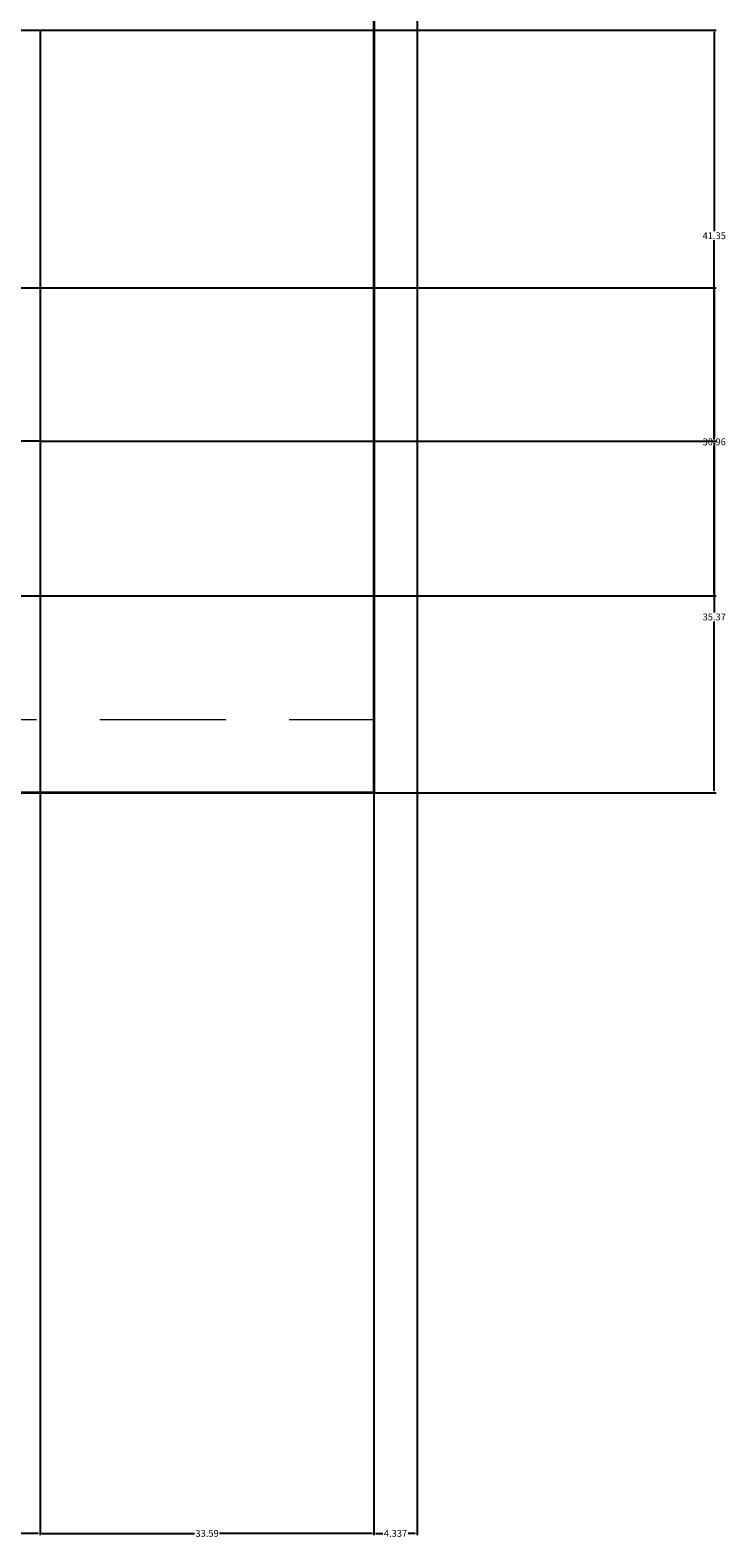
# Model space of a CAD drawing. Units: inches. Extents: x -145 to 510, y 5 to 386.
# Tile 18 of 25: x 440 to 510, y 5 to 157. Entities that reach past the tile are written whole.
import ezdxf

# ---------------------------------------------------------------- set-up
doc = ezdxf.new("R2010")
doc.units = ezdxf.units.IN
doc.header["$MEASUREMENT"] = 0
doc.linetypes.add('DASHED', pattern=[19.05, 12.7, -6.35])
for name, color, linetype, lineweight in [('A-ANNO-DIMS', 2, 'Continuous', 18), ('A-ELEV', 7, 'Continuous', 35), ('A-ELEV-HIDN', 8, 'DASHED', 18), ('A-GLAZ', 4, 'Continuous', 25)]:
    doc.layers.add(name, color=color, linetype=linetype, lineweight=lineweight)
doc.styles.get("Standard").update_dxf_attribs({"font": 'arial.ttf'})
doc.dimstyles.get("Standard").update_dxf_attribs({"dimtxt": 0.6875, "dimasz": 0.18, "dimexe": 0.18, "dimexo": 0.0625, "dimgap": 0.09, "dimtad": 0, "dimtih": 1, "dimtoh": 1, "dimdec": 4, "dimzin": 0, "dimdsep": 46, "dimlunit": 4, "dimtxsty": 'Standard', "dimcen": 0.09, "dimadec": 0, "dimazin": 0, "dimtfac": 1, "dimtdec": 4, "dimtofl": 0, "dimtmove": 0, "dimatfit": 3, "dimfxl": 1, "dimtolj": 1, "dimtzin": 0, "dimarcsym": 0})

# ---------------------------------------------------------------- blocks, each defined once
blk = doc.blocks.new('*D12')
at = {"layer": 'A-ANNO-DIMS', "color": 0, "lineweight": -2, "transparency": 16777216}
for p, q in [((353.23, 115.19), (353.23, 5.19)), ((440.9, 115.19), (440.9, 5.19)), ((353.41, 5.37), (395.82, 5.37)), ((440.72, 5.37), (398.32, 5.37))]:
    blk.add_line(p, q, dxfattribs=at)
at = {"layer": 'A-ANNO-DIMS', "color": 0, "transparency": 16777216}
for points in [[(353.41, 5.4), (353.41, 5.34), (353.23, 5.37)], [(440.72, 5.4), (440.72, 5.34), (440.9, 5.37)]]:
    blk.add_solid(points, dxfattribs=at)
at = {"layer": 'Defpoints', "color": 0, "transparency": 16777216}
for p in [(353.23, 115.26), (440.9, 115.26), (440.9, 5.37)]:
    blk.add_point(p, dxfattribs=at)
at = {"layer": 'A-ANNO-DIMS', "color": 0, "transparency": 16777216, "insert": (397.07, 5.37), "char_height": 0.688, "attachment_point": 5}
blk.add_mtext('\\A1;87.67', dxfattribs=at)
blk = doc.blocks.new('*D13')
at = {"layer": 'A-ANNO-DIMS', "color": 0, "lineweight": -2, "transparency": 16777216}
for p, q in [((440.9, 115.19), (440.9, 5.19)), ((474.49, 79.83), (474.49, 5.19)), ((441.08, 5.37), (456.44, 5.37)), ((474.31, 5.37), (458.95, 5.37))]:
    blk.add_line(p, q, dxfattribs=at)
at = {"layer": 'A-ANNO-DIMS', "color": 0, "transparency": 16777216}
for points in [[(441.08, 5.4), (441.08, 5.34), (440.9, 5.37)], [(474.31, 5.4), (474.31, 5.34), (474.49, 5.37)]]:
    blk.add_solid(points, dxfattribs=at)
at = {"layer": 'Defpoints', "color": 0, "transparency": 16777216}
for p in [(440.9, 115.26), (474.49, 79.89), (474.49, 5.37)]:
    blk.add_point(p, dxfattribs=at)
at = {"layer": 'A-ANNO-DIMS', "color": 0, "transparency": 16777216, "insert": (457.7, 5.37), "char_height": 0.688, "attachment_point": 5}
blk.add_mtext('\\A1;33.59', dxfattribs=at)
blk = doc.blocks.new('*D19')
at = {"layer": 'A-ANNO-DIMS', "color": 0, "lineweight": -2, "transparency": 16777216}
for p, q in [((478.76, 355.89), (-144.05, 355.89)), ((-143.87, 355.71), (-143.87, 218.33)), ((-143.87, 80.07), (-143.87, 217.45)), ((-114.04, 79.89), (-144.05, 79.89))]:
    blk.add_line(p, q, dxfattribs=at)
at = {"layer": 'A-ANNO-DIMS', "color": 0, "transparency": 16777216}
for points in [[(-143.9, 355.71), (-143.84, 355.71), (-143.87, 355.89)], [(-143.9, 80.07), (-143.84, 80.07), (-143.87, 79.89)]]:
    blk.add_solid(points, dxfattribs=at)
at = {"layer": 'Defpoints', "color": 0, "transparency": 16777216}
for p in [(-143.87, 355.89), (478.83, 355.89), (-113.97, 79.89)]:
    blk.add_point(p, dxfattribs=at)
at = {"layer": 'A-ANNO-DIMS', "color": 0, "transparency": 16777216, "insert": (-143.87, 217.89), "char_height": 0.688, "attachment_point": 5}
blk.add_mtext('\\A1;276', dxfattribs=at)
blk = doc.blocks.new('*D31')
at = {"layer": 'A-ANNO-DIMS', "color": 0, "lineweight": -2, "transparency": 16777216}
for p, q in [((440.96, 115.26), (508.91, 115.26)), ((508.73, 115.08), (508.73, 98.02)), ((508.73, 80.07), (508.73, 97.13)), ((474.55, 79.89), (508.91, 79.89))]:
    blk.add_line(p, q, dxfattribs=at)
at = {"layer": 'A-ANNO-DIMS', "color": 0, "transparency": 16777216}
for points in [[(508.7, 115.08), (508.76, 115.08), (508.73, 115.26)], [(508.7, 80.07), (508.76, 80.07), (508.73, 79.89)]]:
    blk.add_solid(points, dxfattribs=at)
at = {"layer": 'Defpoints', "color": 0, "transparency": 16777216}
for p in [(440.9, 115.26), (508.73, 115.26), (474.49, 79.89)]:
    blk.add_point(p, dxfattribs=at)
at = {"layer": 'A-ANNO-DIMS', "color": 0, "transparency": 16777216, "insert": (508.73, 97.57), "char_height": 0.688, "attachment_point": 5}
blk.add_mtext('\\A1;35.37', dxfattribs=at)
blk = doc.blocks.new('*D32')
at = {"layer": 'A-ANNO-DIMS', "color": 0, "lineweight": -2, "transparency": 16777216}
for p, q in [((440.96, 156.61), (508.91, 156.61)), ((508.73, 156.43), (508.73, 136.37)), ((508.73, 115.44), (508.73, 135.49)), ((440.96, 115.26), (508.91, 115.26))]:
    blk.add_line(p, q, dxfattribs=at)
at = {"layer": 'A-ANNO-DIMS', "color": 0, "transparency": 16777216}
for points in [[(508.7, 156.43), (508.76, 156.43), (508.73, 156.61)], [(508.7, 115.44), (508.76, 115.44), (508.73, 115.26)]]:
    blk.add_solid(points, dxfattribs=at)
at = {"layer": 'Defpoints', "color": 0, "transparency": 16777216}
for p in [(440.9, 156.61), (508.73, 156.61), (440.9, 115.26)]:
    blk.add_point(p, dxfattribs=at)
at = {"layer": 'A-ANNO-DIMS', "color": 0, "transparency": 16777216, "insert": (508.73, 135.93), "char_height": 0.688, "attachment_point": 5}
blk.add_mtext('\\A1;41.35', dxfattribs=at)
blk = doc.blocks.new('*D49')
at = {"layer": 'A-ANNO-DIMS', "color": 0, "lineweight": -2, "transparency": 16777216}
for p, q in [((474.49, 223.83), (474.49, 5.19)), ((478.83, 223.83), (478.83, 5.19)), ((474.67, 5.37), (475.39, 5.37)), ((478.65, 5.37), (477.92, 5.37))]:
    blk.add_line(p, q, dxfattribs=at)
at = {"layer": 'A-ANNO-DIMS', "color": 0, "transparency": 16777216}
for points in [[(474.67, 5.4), (474.67, 5.34), (474.49, 5.37)], [(478.65, 5.4), (478.65, 5.34), (478.83, 5.37)]]:
    blk.add_solid(points, dxfattribs=at)
at = {"layer": 'Defpoints', "color": 0, "transparency": 16777216}
for p in [(474.49, 223.89), (478.83, 223.89), (478.83, 5.37)]:
    blk.add_point(p, dxfattribs=at)
at = {"layer": 'A-ANNO-DIMS', "color": 0, "transparency": 16777216, "insert": (476.66, 5.37), "char_height": 0.688, "attachment_point": 5}
blk.add_mtext('\\A1;4.337', dxfattribs=at)
blk = doc.blocks.new('*D58')
at = {"layer": 'A-ANNO-DIMS', "color": 0, "lineweight": -2, "transparency": 16777216}
for p, q in [((265.82, 130.67), (508.91, 130.67)), ((508.73, 130.49), (508.73, 115.63)), ((508.73, 99.89), (508.73, 114.75)), ((265.82, 99.71), (508.91, 99.71))]:
    blk.add_line(p, q, dxfattribs=at)
at = {"layer": 'A-ANNO-DIMS', "color": 0, "transparency": 16777216}
for points in [[(508.7, 130.49), (508.76, 130.49), (508.73, 130.67)], [(508.7, 99.89), (508.76, 99.89), (508.73, 99.71)]]:
    blk.add_solid(points, dxfattribs=at)
at = {"layer": 'Defpoints', "color": 0, "transparency": 16777216}
for p in [(265.76, 130.67), (508.73, 130.67), (265.76, 99.71)]:
    blk.add_point(p, dxfattribs=at)
at = {"layer": 'A-ANNO-DIMS', "color": 0, "transparency": 16777216, "insert": (508.73, 115.19), "char_height": 0.688, "attachment_point": 5}
blk.add_mtext('\\A1;30.96', dxfattribs=at)

msp = doc.modelspace()

# ---------------------------------------------------------------- linework, layer by layer
at = {"layer": 'A-ELEV'}
for p, q in [((474.4893, 223.8905), (474.4893, 79.8905)), ((474.4893, 79.8905), (392.4492, 79.8905))]:
    msp.add_line(p, q, dxfattribs=at)
at = {"layer": 'A-ELEV-HIDN'}
msp.add_line((313.5545, 87.2638), (474.4893, 87.2638), dxfattribs=at)
at = {"layer": 'A-GLAZ'}
msp.add_lwpolyline([(353.234, 156.6093), (440.9009, 156.6093), (440.9009, 115.2574), (353.234, 115.2574)], close=True, dxfattribs=at)

# ---------------------------------------------------------------- dimensions: what is measured, and where the dimension line sits
at = {"layer": 'A-ANNO-DIMS'}
for base, p1, p2, override, picture, middle in [((-143.8737, 355.8905), (-113.9737, 79.8905), (478.8263, 355.8905), {"dimdec": 0, "dimlfac": 1, "dimrnd": 0, "dimzin": 0, "dimdsep": 46, "dimlunit": 2}, '*D19', (-143.8737, 217.8905)), ((508.7263, 156.6093), (440.9009, 115.2574), (440.9009, 156.6093), {"dimdec": 2, "dimlfac": 1, "dimrnd": 0, "dimzin": 0, "dimdsep": 46, "dimlunit": 2}, '*D32', (508.7263, 135.9333)), ((508.7263, 130.6707), (265.7612, 99.7118), (265.7612, 130.6707), {"dimdec": 2, "dimlfac": 1, "dimrnd": 0, "dimzin": 0, "dimdsep": 46, "dimlunit": 2}, '*D58', (508.7263, 115.1912)), ((508.7263, 115.2574), (474.4893, 79.8905), (440.9009, 115.2574), {"dimdec": 2, "dimlfac": 1, "dimrnd": 0, "dimzin": 0, "dimdsep": 46, "dimlunit": 2}, '*D31', (508.7263, 97.574))]:
    dim = msp.add_linear_dim(base=base, p1=p1, p2=p2, angle=90, dimstyle='Standard', override=override, dxfattribs=at)
    dim.commit()
    dim.dimension.update_dxf_attribs({"geometry": picture, "text_midpoint": middle})
for base, p1, p2, override, picture, middle in [((478.8263, 5.3738), (474.4893, 223.8905), (478.8263, 223.8905), {"dimdec": 3, "dimlfac": 1, "dimrnd": 0, "dimzin": 0, "dimdsep": 46, "dimlunit": 2}, '*D49', (476.6578, 5.3738)), ((440.9009, 5.3738), (353.234, 115.2574), (440.9009, 115.2574), {"dimdec": 2, "dimlfac": 1, "dimrnd": 0, "dimzin": 0, "dimdsep": 46, "dimlunit": 2}, '*D12', (397.0675, 5.3738)), ((474.4893, 5.3738), (440.9009, 115.2574), (474.4893, 79.8905), {"dimdec": 2, "dimlfac": 1, "dimrnd": 0, "dimzin": 0, "dimdsep": 46, "dimlunit": 2}, '*D13', (457.6951, 5.3738))]:
    dim = msp.add_linear_dim(base=base, p1=p1, p2=p2, dimstyle='Standard', override=override, dxfattribs=at)
    dim.commit()
    dim.dimension.update_dxf_attribs({"geometry": picture, "text_midpoint": middle})

doc.saveas('drawing.dxf')
